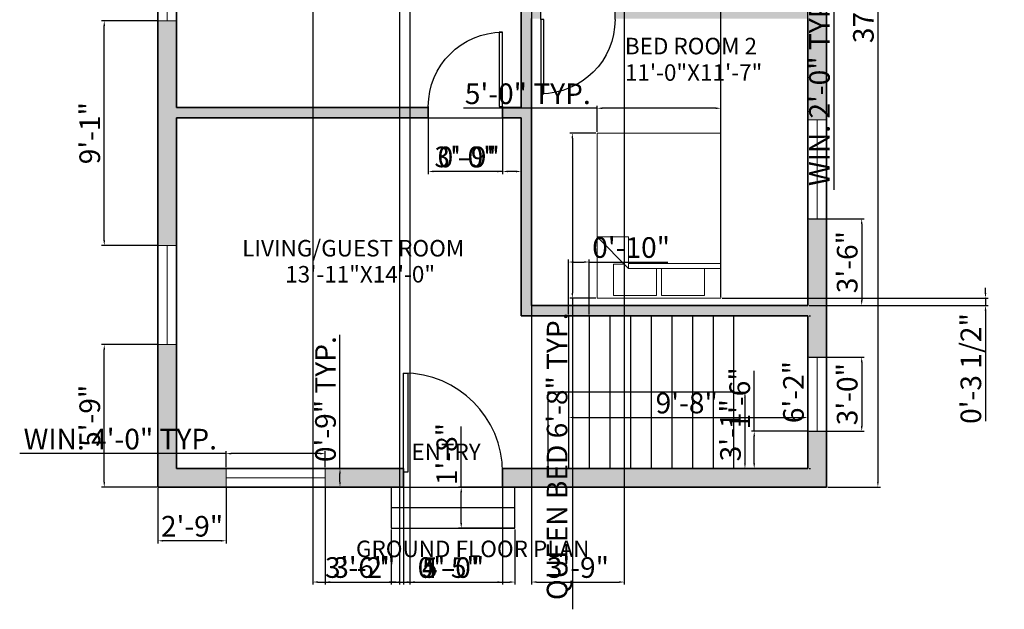
# Model space of a CAD drawing. Units: inches. Extents: x 3647 to 4124, y 1633 to 2205.
# Tile 1 of 3: x 3647 to 4124, y 1633 to 1919. Entities that reach past the tile are written whole.
import ezdxf

# ---------------------------------------------------------------- set-up
doc = ezdxf.new("R2010")
doc.units = ezdxf.units.IN
for name, color, linetype, lineweight in [('A-ANNO-DIMS', 2, 'Continuous', 18), ('A-ANNO-TEXT', 3, 'Continuous', 25), ('A-AREA-IDEN', 3, 'Continuous', 18), ('A-FURN', 8, 'Continuous', 18), ('DOOR', 6, 'Continuous', 25), ('STAIRS', 1, 'Continuous', 25), ('WALL', 42, 'Continuous', 35), ('WINDOW', 4, 'Continuous', 18)]:
    doc.layers.add(name, color=color, linetype=linetype, lineweight=lineweight)
doc.layers.add('A-WALL-PATT', color=18, linetype='Continuous', lineweight=13, true_color=0x000000)
doc.styles.get("Standard").update_dxf_attribs({"font": 'arial.ttf'})
doc.dimstyles.new('ISO-25', dxfattribs={"dimtxt": 10, "dimasz": 2.5, "dimexe": 1.25, "dimexo": 0.625, "dimtad": 1, "dimdec": 1, "dimlunit": 3, "dimtxsty": 'Standard', "dimcen": 2.5, "dimadec": 0, "dimazin": 0, "dimtfac": 1, "dimtdec": 1, "dimtmove": 0, "dimatfit": 3, "dimfxl": 1, "dimarcsym": 0})

# ---------------------------------------------------------------- blocks, each defined once
blk = doc.blocks.new('*U2')
for p, q in [((0, 0), (0, -6)), ((40, 0), (40, -6))]:
    blk.add_line(p, q)
blk.add_lwpolyline([(0, 0), (0, 40), (1.75, 40), (1.75, 0)], close=True)
blk.add_arc((0, 0), 40, 0, 90)
blk = doc.blocks.new('Bed - Queen')
for p, q in [((0, -80.00003), (0, 0)), ((0, 0), (59.99999, 0)), ((59.99999, 0), (59.99999, -80.00003)), ((7.99999, -1.2), (28.79998, -1.2)), ((7.99999, -14.4), (7.99999, -1.2)), ((28.79998, -1.2), (28.79998, -14.4)), ((31.19999, -1.2), (51.99999, -1.2)), ((31.19999, -14.4), (31.19999, -1.2)), ((51.99999, -1.2), (51.99999, -16.4)), ((0, -14.4), (44.8, -14.4)), ((44.8, -16.8), (0, -16.8)), ((59.99999, -29.6), (44.8, -14.4)), ((44.8, -14.4), (44.8, -29.6)), ((51.99999, -16.4), (46.79936, -16.4)), ((44.8, -29.6), (59.99999, -29.6)), ((59.99999, -80.00003), (0, -80.00003))]:
    blk.add_line(p, q)
blk = doc.blocks.new('*D8')
at = {"layer": 'A-ANNO-DIMS', "color": 0, "lineweight": -2, "transparency": 16777216}
for p, q in [((4029.34, 1775.28), (4029.96, 1775.28)), ((4028.71, 1772.78), (4028.71, 1703.78)), ((4029.34, 1701.28), (4029.96, 1701.28))]:
    blk.add_line(p, q, dxfattribs=at)
at = {"layer": 'A-ANNO-DIMS', "color": 0, "transparency": 16777216}
for points in [[(4028.3, 1772.78), (4029.13, 1772.78), (4028.71, 1775.28)], [(4028.3, 1703.78), (4029.13, 1703.78), (4028.71, 1701.28)]]:
    blk.add_solid(points, dxfattribs=at)
at = {"layer": 'Defpoints', "color": 0, "transparency": 16777216}
for p in [(4028.71, 1775.28), (4028.71, 1701.28), (4028.71, 1701.28)]:
    blk.add_point(p, dxfattribs=at)
at = {"layer": 'A-ANNO-DIMS', "color": 0, "transparency": 16777216, "insert": (4022.98, 1738.28), "char_height": 10, "attachment_point": 5, "rotation": 90}
blk.add_mtext('6\'-2"', dxfattribs=at)
blk = doc.blocks.new('*D9')
at = {"layer": 'A-ANNO-DIMS', "color": 0, "lineweight": -2, "transparency": 16777216}
for p, q in [((3912.71, 1737.66), (3912.71, 1724.71)), ((4028.71, 1737.66), (4028.71, 1724.71)), ((3915.21, 1725.96), (4026.21, 1725.96))]:
    blk.add_line(p, q, dxfattribs=at)
at = {"layer": 'A-ANNO-DIMS', "color": 0, "transparency": 16777216}
for points in [[(3915.21, 1726.38), (3915.21, 1725.54), (3912.71, 1725.96)], [(4026.21, 1726.38), (4026.21, 1725.54), (4028.71, 1725.96)]]:
    blk.add_solid(points, dxfattribs=at)
at = {"layer": 'Defpoints', "color": 0, "transparency": 16777216}
for p in [(3912.71, 1738.28), (4028.71, 1738.28), (4028.71, 1725.96)]:
    blk.add_point(p, dxfattribs=at)
at = {"layer": 'A-ANNO-DIMS', "color": 0, "transparency": 16777216, "insert": (3969.95, 1731.69), "char_height": 10, "attachment_point": 5}
blk.add_mtext('9\'-8"', dxfattribs=at)
blk = doc.blocks.new('*D10')
at = {"layer": 'A-ANNO-DIMS', "color": 0, "lineweight": -2, "transparency": 16777216}
for p, q in [((3993.34, 1738.28), (3999.44, 1738.28)), ((3998.19, 1735.78), (3998.19, 1703.78)), ((3993.34, 1701.28), (3999.44, 1701.28))]:
    blk.add_line(p, q, dxfattribs=at)
at = {"layer": 'A-ANNO-DIMS', "color": 0, "transparency": 16777216}
for points in [[(3997.78, 1735.78), (3998.61, 1735.78), (3998.19, 1738.28)], [(3997.78, 1703.78), (3998.61, 1703.78), (3998.19, 1701.28)]]:
    blk.add_solid(points, dxfattribs=at)
at = {"layer": 'Defpoints', "color": 0, "transparency": 16777216}
for p in [(3992.71, 1738.28), (3992.71, 1701.28), (3998.19, 1701.28)]:
    blk.add_point(p, dxfattribs=at)
at = {"layer": 'A-ANNO-DIMS', "color": 0, "transparency": 16777216, "insert": (3992.46, 1719.78), "char_height": 10, "attachment_point": 5, "rotation": 90}
blk.add_mtext('3\'-1"', dxfattribs=at)
blk = doc.blocks.new('*D12')
at = {"layer": 'A-ANNO-DIMS', "color": 0, "lineweight": -2, "transparency": 16777216}
for p, q in [((4038.34, 2136.28), (4063.86, 2136.28)), ((4062.61, 2133.78), (4062.61, 1694.78)), ((4038.34, 1692.28), (4063.86, 1692.28))]:
    blk.add_line(p, q, dxfattribs=at)
at = {"layer": 'A-ANNO-DIMS', "color": 0, "transparency": 16777216}
for points in [[(4062.19, 2133.78), (4063.02, 2133.78), (4062.61, 2136.28)], [(4062.19, 1694.78), (4063.02, 1694.78), (4062.61, 1692.28)]]:
    blk.add_solid(points, dxfattribs=at)
at = {"layer": 'Defpoints', "color": 0, "transparency": 16777216}
for p in [(4037.71, 2136.28), (4037.71, 1692.28), (4062.61, 1692.28)]:
    blk.add_point(p, dxfattribs=at)
at = {"layer": 'A-ANNO-DIMS', "color": 0, "transparency": 16777216, "insert": (4056.87, 1916.88), "char_height": 10, "attachment_point": 5, "rotation": 90}
blk.add_mtext("37'", dxfattribs=at)
blk = doc.blocks.new('WIN-48IN')
for p, q in [((9, 48), (0, 48)), ((4.5, 48), (4.5, 0)), ((9, 0), (0, 0))]:
    blk.add_line(p, q)
blk = doc.blocks.new('*D15')
at = {"layer": 'A-ANNO-DIMS', "color": 0, "lineweight": -2, "transparency": 16777216}
for p, q in [((3746.71, 1708.48), (3646.68, 1708.48)), ((3746.71, 1701.91), (3746.71, 1709.73)), ((3792.21, 1708.48), (3749.21, 1708.48)), ((3794.71, 1701.91), (3794.71, 1709.73))]:
    blk.add_line(p, q, dxfattribs=at)
at = {"layer": 'A-ANNO-DIMS', "color": 0, "transparency": 16777216}
for points in [[(3749.21, 1708.9), (3749.21, 1708.06), (3746.71, 1708.48)], [(3792.21, 1708.9), (3792.21, 1708.06), (3794.71, 1708.48)]]:
    blk.add_solid(points, dxfattribs=at)
at = {"layer": 'Defpoints', "color": 0, "transparency": 16777216}
for p in [(3746.71, 1708.48), (3746.71, 1701.28), (3794.71, 1701.28)]:
    blk.add_point(p, dxfattribs=at)
at = {"layer": 'A-ANNO-DIMS', "color": 0, "transparency": 16777216, "insert": (3695.45, 1714.21), "char_height": 10, "attachment_point": 5}
blk.add_mtext('WIN. 4\'-0" TYP.', dxfattribs=at)
blk = doc.blocks.new('*D16')
at = {"layer": 'A-ANNO-DIMS', "color": 0, "lineweight": -2, "transparency": 16777216}
for p, q in [((3801.91, 1701.28), (3801.91, 1765.99)), ((3795.34, 1701.28), (3803.16, 1701.28)), ((3801.91, 1694.78), (3801.91, 1698.78)), ((3795.34, 1692.28), (3803.16, 1692.28))]:
    blk.add_line(p, q, dxfattribs=at)
at = {"layer": 'A-ANNO-DIMS', "color": 0, "transparency": 16777216}
for points in [[(3801.5, 1698.78), (3802.33, 1698.78), (3801.91, 1701.28)], [(3801.5, 1694.78), (3802.33, 1694.78), (3801.91, 1692.28)]]:
    blk.add_solid(points, dxfattribs=at)
at = {"layer": 'Defpoints', "color": 0, "transparency": 16777216}
for p in [(3794.71, 1701.28), (3801.91, 1701.28), (3794.71, 1692.28)]:
    blk.add_point(p, dxfattribs=at)
at = {"layer": 'A-ANNO-DIMS', "color": 0, "transparency": 16777216, "insert": (3796.18, 1734.88), "char_height": 10, "attachment_point": 5, "rotation": 90}
blk.add_mtext('0\'-9" TYP.', dxfattribs=at)
blk = doc.blocks.new('*D17')
at = {"layer": 'A-ANNO-DIMS', "color": 0, "lineweight": -2, "transparency": 16777216}
for p, q in [((4038.34, 1960.28), (4042.56, 1960.28)), ((4041.31, 1957.78), (4041.31, 1938.78)), ((4038.34, 1936.28), (4042.56, 1936.28)), ((4041.31, 1936.28), (4041.31, 1836.25))]:
    blk.add_line(p, q, dxfattribs=at)
at = {"layer": 'A-ANNO-DIMS', "color": 0, "transparency": 16777216}
for points in [[(4040.9, 1957.78), (4041.73, 1957.78), (4041.31, 1960.28)], [(4040.9, 1938.78), (4041.73, 1938.78), (4041.31, 1936.28)]]:
    blk.add_solid(points, dxfattribs=at)
at = {"layer": 'Defpoints', "color": 0, "transparency": 16777216}
for p in [(4037.71, 1960.28), (4037.71, 1936.28), (4041.31, 1936.28)]:
    blk.add_point(p, dxfattribs=at)
at = {"layer": 'A-ANNO-DIMS', "color": 0, "transparency": 16777216, "insert": (4035.58, 1885.02), "char_height": 10, "attachment_point": 5, "rotation": 90}
blk.add_mtext('WIN. 2\'-0" TYP.', dxfattribs=at)
blk = doc.blocks.new('*D19')
at = {"layer": 'A-ANNO-DIMS', "color": 0, "lineweight": -2, "transparency": 16777216}
for p, q in [((3925.91, 1863.86), (3913.28, 1863.86)), ((3914.53, 1861.36), (3914.53, 1786.36)), ((3925.91, 1783.86), (3913.28, 1783.86)), ((3914.53, 1783.86), (3914.53, 1633.01))]:
    blk.add_line(p, q, dxfattribs=at)
at = {"layer": 'A-ANNO-DIMS', "color": 0, "transparency": 16777216}
for points in [[(3914.12, 1861.36), (3914.95, 1861.36), (3914.53, 1863.86)], [(3914.12, 1786.36), (3914.95, 1786.36), (3914.53, 1783.86)]]:
    blk.add_solid(points, dxfattribs=at)
at = {"layer": 'Defpoints', "color": 0, "transparency": 16777216}
for p in [(3926.53, 1863.86), (3914.53, 1783.86), (3926.53, 1783.86)]:
    blk.add_point(p, dxfattribs=at)
at = {"layer": 'A-ANNO-DIMS', "color": 0, "transparency": 16777216, "insert": (3908.43, 1707.19), "char_height": 10, "attachment_point": 5, "rotation": 90}
blk.add_mtext('QUEEN BED 6\'-8" TYP.', dxfattribs=at)
blk = doc.blocks.new('*D20')
at = {"layer": 'A-ANNO-DIMS', "color": 0, "lineweight": -2, "transparency": 16777216}
for p, q in [((3926.53, 1875.86), (3861.83, 1875.86)), ((3926.53, 1864.49), (3926.53, 1877.11)), ((3984.03, 1875.86), (3929.03, 1875.86)), ((3986.53, 1864.49), (3986.53, 1877.11))]:
    blk.add_line(p, q, dxfattribs=at)
at = {"layer": 'A-ANNO-DIMS', "color": 0, "transparency": 16777216}
for points in [[(3929.03, 1876.28), (3929.03, 1875.45), (3926.53, 1875.86)], [(3984.03, 1876.28), (3984.03, 1875.45), (3986.53, 1875.86)]]:
    blk.add_solid(points, dxfattribs=at)
at = {"layer": 'Defpoints', "color": 0, "transparency": 16777216}
for p in [(3926.53, 1875.86), (3926.53, 1863.86), (3986.53, 1863.86)]:
    blk.add_point(p, dxfattribs=at)
at = {"layer": 'A-ANNO-DIMS', "color": 0, "transparency": 16777216, "insert": (3892.93, 1881.59), "char_height": 10, "attachment_point": 5}
blk.add_mtext('5\'-0" TYP.', dxfattribs=at)
blk = doc.blocks.new('*D28')
at = {"layer": 'A-ANNO-DIMS', "color": 0, "lineweight": -2, "transparency": 16777216}
for p, q in [((3844.71, 1870.66), (3844.71, 1843.98)), ((3880.71, 1870.66), (3880.71, 1843.98)), ((3878.21, 1845.23), (3847.21, 1845.23))]:
    blk.add_line(p, q, dxfattribs=at)
at = {"layer": 'A-ANNO-DIMS', "color": 0, "transparency": 16777216}
for points in [[(3847.21, 1845.65), (3847.21, 1844.81), (3844.71, 1845.23)], [(3878.21, 1845.65), (3878.21, 1844.81), (3880.71, 1845.23)]]:
    blk.add_solid(points, dxfattribs=at)
at = {"layer": 'Defpoints', "color": 0, "transparency": 16777216}
for p in [(3844.71, 1871.28), (3880.71, 1871.28), (3844.71, 1845.23)]:
    blk.add_point(p, dxfattribs=at)
at = {"layer": 'A-ANNO-DIMS', "color": 0, "transparency": 16777216, "insert": (3862.71, 1850.97), "char_height": 10, "attachment_point": 5}
blk.add_mtext('3\'-0"', dxfattribs=at)
blk = doc.blocks.new('*D30')
at = {"layer": 'A-ANNO-DIMS', "color": 0, "lineweight": -2, "transparency": 16777216}
for p, q in [((3894.71, 1989.66), (3894.71, 1644.98)), ((3939.71, 1989.66), (3939.71, 1644.98)), ((3897.21, 1646.23), (3937.21, 1646.23))]:
    blk.add_line(p, q, dxfattribs=at)
at = {"layer": 'A-ANNO-DIMS', "color": 0, "transparency": 16777216}
for points in [[(3897.21, 1646.65), (3897.21, 1645.81), (3894.71, 1646.23)], [(3937.21, 1646.65), (3937.21, 1645.81), (3939.71, 1646.23)]]:
    blk.add_solid(points, dxfattribs=at)
at = {"layer": 'Defpoints', "color": 0, "transparency": 16777216}
for p in [(3894.71, 1990.28), (3939.71, 1990.28), (3939.71, 1646.23)]:
    blk.add_point(p, dxfattribs=at)
at = {"layer": 'A-ANNO-DIMS', "color": 0, "transparency": 16777216, "insert": (3917.21, 1651.97), "char_height": 10, "attachment_point": 5}
blk.add_mtext('3\'-9"', dxfattribs=at)
blk = doc.blocks.new('*D31')
at = {"layer": 'A-ANNO-DIMS', "color": 0, "lineweight": -2, "transparency": 16777216}
for p, q in [((3788.71, 2013.66), (3788.71, 1644.98)), ((3830.71, 2013.66), (3830.71, 1644.98)), ((3791.21, 1646.23), (3828.21, 1646.23))]:
    blk.add_line(p, q, dxfattribs=at)
at = {"layer": 'A-ANNO-DIMS', "color": 0, "transparency": 16777216}
for points in [[(3791.21, 1646.65), (3791.21, 1645.81), (3788.71, 1646.23)], [(3828.21, 1646.65), (3828.21, 1645.81), (3830.71, 1646.23)]]:
    blk.add_solid(points, dxfattribs=at)
at = {"layer": 'Defpoints', "color": 0, "transparency": 16777216}
for p in [(3788.71, 2014.28), (3830.71, 2014.28), (3830.71, 1646.23)]:
    blk.add_point(p, dxfattribs=at)
at = {"layer": 'A-ANNO-DIMS', "color": 0, "transparency": 16777216, "insert": (3809.71, 1651.97), "char_height": 10, "attachment_point": 5}
blk.add_mtext('3\'-6"', dxfattribs=at)
blk = doc.blocks.new('*D32')
at = {"layer": 'A-ANNO-DIMS', "color": 0, "lineweight": -2, "transparency": 16777216}
for p, q in [((3830.71, 2126.66), (3830.71, 1644.98)), ((3835.71, 2126.66), (3835.71, 1644.98)), ((3828.21, 1646.23), (3825.71, 1646.23)), ((3830.71, 1646.23), (3835.71, 1646.23)), ((3838.21, 1646.23), (3868.55, 1646.23))]:
    blk.add_line(p, q, dxfattribs=at)
at = {"layer": 'A-ANNO-DIMS', "color": 0, "transparency": 16777216}
for points in [[(3828.21, 1646.65), (3828.21, 1645.81), (3830.71, 1646.23)], [(3838.21, 1646.65), (3838.21, 1645.81), (3835.71, 1646.23)]]:
    blk.add_solid(points, dxfattribs=at)
at = {"layer": 'Defpoints', "color": 0, "transparency": 16777216}
for p in [(3830.71, 2127.28), (3835.71, 2127.28), (3835.71, 1646.23)]:
    blk.add_point(p, dxfattribs=at)
at = {"layer": 'A-ANNO-DIMS', "color": 0, "transparency": 16777216, "insert": (3854.63, 1651.96), "char_height": 10, "attachment_point": 5}
blk.add_mtext('0\'-5"', dxfattribs=at)
blk = doc.blocks.new('*D33')
at = {"layer": 'A-ANNO-DIMS', "color": 0, "lineweight": -2, "transparency": 16777216}
for p, q in [((3713.71, 1691.66), (3713.71, 1664.98)), ((3746.71, 1691.66), (3746.71, 1664.98)), ((3744.21, 1666.23), (3716.21, 1666.23))]:
    blk.add_line(p, q, dxfattribs=at)
at = {"layer": 'A-ANNO-DIMS', "color": 0, "transparency": 16777216}
for points in [[(3716.21, 1666.65), (3716.21, 1665.81), (3713.71, 1666.23)], [(3744.21, 1666.65), (3744.21, 1665.81), (3746.71, 1666.23)]]:
    blk.add_solid(points, dxfattribs=at)
at = {"layer": 'Defpoints', "color": 0, "transparency": 16777216}
for p in [(3713.71, 1692.28), (3746.71, 1692.28), (3713.71, 1666.23)]:
    blk.add_point(p, dxfattribs=at)
at = {"layer": 'A-ANNO-DIMS', "color": 0, "transparency": 16777216, "insert": (3730.21, 1671.96), "char_height": 10, "attachment_point": 5}
blk.add_mtext('2\'-9"', dxfattribs=at)
blk = doc.blocks.new('*D34')
at = {"layer": 'A-ANNO-DIMS', "color": 0, "lineweight": -2, "transparency": 16777216}
for p, q in [((3794.71, 1691.66), (3794.71, 1644.98)), ((3832.71, 1691.66), (3832.71, 1644.98)), ((3797.21, 1646.23), (3830.21, 1646.23))]:
    blk.add_line(p, q, dxfattribs=at)
at = {"layer": 'A-ANNO-DIMS', "color": 0, "transparency": 16777216}
for points in [[(3797.21, 1646.65), (3797.21, 1645.81), (3794.71, 1646.23)], [(3830.21, 1646.65), (3830.21, 1645.81), (3832.71, 1646.23)]]:
    blk.add_solid(points, dxfattribs=at)
at = {"layer": 'Defpoints', "color": 0, "transparency": 16777216}
for p in [(3794.71, 1692.28), (3832.71, 1692.28), (3832.71, 1646.23)]:
    blk.add_point(p, dxfattribs=at)
at = {"layer": 'A-ANNO-DIMS', "color": 0, "transparency": 16777216, "insert": (3813.71, 1651.97), "char_height": 10, "attachment_point": 5}
blk.add_mtext('3\'-2"', dxfattribs=at)
blk = doc.blocks.new('*D35')
at = {"layer": 'A-ANNO-DIMS', "color": 0, "lineweight": -2, "transparency": 16777216}
for p, q in [((3832.71, 1691.66), (3832.71, 1644.98)), ((3880.71, 1691.66), (3880.71, 1644.98)), ((3835.21, 1646.23), (3878.21, 1646.23))]:
    blk.add_line(p, q, dxfattribs=at)
at = {"layer": 'A-ANNO-DIMS', "color": 0, "transparency": 16777216}
for points in [[(3835.21, 1646.65), (3835.21, 1645.81), (3832.71, 1646.23)], [(3878.21, 1646.65), (3878.21, 1645.81), (3880.71, 1646.23)]]:
    blk.add_solid(points, dxfattribs=at)
at = {"layer": 'Defpoints', "color": 0, "transparency": 16777216}
for p in [(3832.71, 1692.28), (3880.71, 1692.28), (3880.71, 1646.23)]:
    blk.add_point(p, dxfattribs=at)
at = {"layer": 'A-ANNO-DIMS', "color": 0, "transparency": 16777216, "insert": (3856.71, 1651.96), "char_height": 10, "attachment_point": 5}
blk.add_mtext('4\'-0"', dxfattribs=at)
blk = doc.blocks.new('*D36')
at = {"layer": 'A-ANNO-DIMS', "color": 0, "lineweight": -2, "transparency": 16777216}
for p, q in [((3826.71, 1671.66), (3826.71, 1644.98)), ((3886.71, 1671.66), (3886.71, 1644.98)), ((3829.21, 1646.23), (3884.21, 1646.23))]:
    blk.add_line(p, q, dxfattribs=at)
at = {"layer": 'A-ANNO-DIMS', "color": 0, "transparency": 16777216}
for points in [[(3829.21, 1646.65), (3829.21, 1645.81), (3826.71, 1646.23)], [(3884.21, 1646.65), (3884.21, 1645.81), (3886.71, 1646.23)]]:
    blk.add_solid(points, dxfattribs=at)
at = {"layer": 'Defpoints', "color": 0, "transparency": 16777216}
for p in [(3826.71, 1672.28), (3886.71, 1672.28), (3886.71, 1646.23)]:
    blk.add_point(p, dxfattribs=at)
at = {"layer": 'A-ANNO-DIMS', "color": 0, "transparency": 16777216, "insert": (3856.71, 1651.96), "char_height": 10, "attachment_point": 5}
blk.add_mtext('5\'-0"', dxfattribs=at)
blk = doc.blocks.new('*D37')
at = {"layer": 'A-ANNO-DIMS', "color": 0, "lineweight": -2, "transparency": 16777216}
for p, q in [((3860.66, 1692.28), (3860.66, 1721.67)), ((3886.09, 1692.28), (3859.41, 1692.28)), ((3860.66, 1674.78), (3860.66, 1689.78)), ((3886.09, 1672.28), (3859.41, 1672.28))]:
    blk.add_line(p, q, dxfattribs=at)
at = {"layer": 'A-ANNO-DIMS', "color": 0, "transparency": 16777216}
for points in [[(3860.25, 1689.78), (3861.08, 1689.78), (3860.66, 1692.28)], [(3860.25, 1674.78), (3861.08, 1674.78), (3860.66, 1672.28)]]:
    blk.add_solid(points, dxfattribs=at)
at = {"layer": 'Defpoints', "color": 0, "transparency": 16777216}
for p in [(3860.66, 1692.28), (3886.71, 1692.28), (3886.71, 1672.28)]:
    blk.add_point(p, dxfattribs=at)
at = {"layer": 'A-ANNO-DIMS', "color": 0, "transparency": 16777216, "insert": (3854.93, 1708.23), "char_height": 10, "attachment_point": 5, "rotation": 90}
blk.add_mtext('1\'-8"', dxfattribs=at)
blk = doc.blocks.new('*D38')
at = {"layer": 'A-ANNO-DIMS', "color": 0, "lineweight": -2, "transparency": 16777216}
for p, q in [((3713.09, 1761.28), (3686.41, 1761.28)), ((3687.66, 1694.78), (3687.66, 1758.78)), ((3713.09, 1692.28), (3686.41, 1692.28))]:
    blk.add_line(p, q, dxfattribs=at)
at = {"layer": 'A-ANNO-DIMS', "color": 0, "transparency": 16777216}
for points in [[(3687.25, 1758.78), (3688.08, 1758.78), (3687.66, 1761.28)], [(3687.25, 1694.78), (3688.08, 1694.78), (3687.66, 1692.28)]]:
    blk.add_solid(points, dxfattribs=at)
at = {"layer": 'Defpoints', "color": 0, "transparency": 16777216}
for p in [(3687.66, 1761.28), (3713.71, 1761.28), (3713.71, 1692.28)]:
    blk.add_point(p, dxfattribs=at)
at = {"layer": 'A-ANNO-DIMS', "color": 0, "transparency": 16777216, "insert": (3681.93, 1726.78), "char_height": 10, "attachment_point": 5, "rotation": 90}
blk.add_mtext('5\'-9"', dxfattribs=at)
blk = doc.blocks.new('*D39')
at = {"layer": 'A-ANNO-DIMS', "color": 0, "lineweight": -2, "transparency": 16777216}
for p, q in [((3713.09, 1918.28), (3686.41, 1918.28)), ((3687.66, 1811.78), (3687.66, 1915.78)), ((3713.09, 1809.28), (3686.41, 1809.28))]:
    blk.add_line(p, q, dxfattribs=at)
at = {"layer": 'A-ANNO-DIMS', "color": 0, "transparency": 16777216}
for points in [[(3687.25, 1915.78), (3688.08, 1915.78), (3687.66, 1918.28)], [(3687.25, 1811.78), (3688.08, 1811.78), (3687.66, 1809.28)]]:
    blk.add_solid(points, dxfattribs=at)
at = {"layer": 'Defpoints', "color": 0, "transparency": 16777216}
for p in [(3687.66, 1918.28), (3713.71, 1918.28), (3713.71, 1809.28)]:
    blk.add_point(p, dxfattribs=at)
at = {"layer": 'A-ANNO-DIMS', "color": 0, "transparency": 16777216, "insert": (3681.93, 1863.78), "char_height": 10, "attachment_point": 5, "rotation": 90}
blk.add_mtext('9\'-1"', dxfattribs=at)
blk = doc.blocks.new('*D44')
at = {"layer": 'A-ANNO-DIMS', "color": 0, "lineweight": -2, "transparency": 16777216}
for p, q in [((4029.34, 1822.28), (4056.01, 1822.28)), ((4054.76, 1819.78), (4054.76, 1782.78)), ((4029.34, 1780.28), (4056.01, 1780.28))]:
    blk.add_line(p, q, dxfattribs=at)
at = {"layer": 'A-ANNO-DIMS', "color": 0, "transparency": 16777216}
for points in [[(4054.35, 1819.78), (4055.18, 1819.78), (4054.76, 1822.28)], [(4054.35, 1782.78), (4055.18, 1782.78), (4054.76, 1780.28)]]:
    blk.add_solid(points, dxfattribs=at)
at = {"layer": 'Defpoints', "color": 0, "transparency": 16777216}
for p in [(4028.71, 1822.28), (4028.71, 1780.28), (4054.76, 1780.28)]:
    blk.add_point(p, dxfattribs=at)
at = {"layer": 'A-ANNO-DIMS', "color": 0, "transparency": 16777216, "insert": (4049.03, 1801.28), "char_height": 10, "attachment_point": 5, "rotation": 90}
blk.add_mtext('3\'-6"', dxfattribs=at)
blk = doc.blocks.new('*D45')
at = {"layer": 'A-ANNO-DIMS', "color": 0, "lineweight": -2, "transparency": 16777216}
for p, q in [((4002.66, 1719.28), (4002.66, 1748.67)), ((4028.09, 1719.28), (4001.41, 1719.28)), ((4002.66, 1703.78), (4002.66, 1716.78)), ((4028.09, 1701.28), (4001.41, 1701.28))]:
    blk.add_line(p, q, dxfattribs=at)
at = {"layer": 'A-ANNO-DIMS', "color": 0, "transparency": 16777216}
for points in [[(4002.25, 1716.78), (4003.08, 1716.78), (4002.66, 1719.28)], [(4002.25, 1703.78), (4003.08, 1703.78), (4002.66, 1701.28)]]:
    blk.add_solid(points, dxfattribs=at)
at = {"layer": 'Defpoints', "color": 0, "transparency": 16777216}
for p in [(4002.66, 1719.28), (4028.71, 1719.28), (4028.71, 1701.28)]:
    blk.add_point(p, dxfattribs=at)
at = {"layer": 'A-ANNO-DIMS', "color": 0, "transparency": 16777216, "insert": (3996.93, 1735.23), "char_height": 10, "attachment_point": 5, "rotation": 90}
blk.add_mtext('1\'-6"', dxfattribs=at)
blk = doc.blocks.new('*D46')
at = {"layer": 'A-ANNO-DIMS', "color": 0, "lineweight": -2, "transparency": 16777216}
for p, q in [((4029.34, 1755.28), (4056.01, 1755.28)), ((4054.76, 1752.78), (4054.76, 1721.78)), ((4029.34, 1719.28), (4056.01, 1719.28))]:
    blk.add_line(p, q, dxfattribs=at)
at = {"layer": 'A-ANNO-DIMS', "color": 0, "transparency": 16777216}
for points in [[(4054.35, 1752.78), (4055.18, 1752.78), (4054.76, 1755.28)], [(4054.35, 1721.78), (4055.18, 1721.78), (4054.76, 1719.28)]]:
    blk.add_solid(points, dxfattribs=at)
at = {"layer": 'Defpoints', "color": 0, "transparency": 16777216}
for p in [(4028.71, 1755.28), (4028.71, 1719.28), (4054.76, 1719.28)]:
    blk.add_point(p, dxfattribs=at)
at = {"layer": 'A-ANNO-DIMS', "color": 0, "transparency": 16777216, "insert": (4049.03, 1737.28), "char_height": 10, "attachment_point": 5, "rotation": 90}
blk.add_mtext('3\'-0"', dxfattribs=at)
blk = doc.blocks.new('*D47')
at = {"layer": 'A-ANNO-DIMS', "color": 0, "lineweight": -2, "transparency": 16777216}
for p, q in [((3880.71, 1870.66), (3880.71, 1843.98)), ((3889.71, 1870.66), (3889.71, 1843.98)), ((3880.71, 1845.23), (3850.38, 1845.23)), ((3887.21, 1845.23), (3883.21, 1845.23))]:
    blk.add_line(p, q, dxfattribs=at)
at = {"layer": 'A-ANNO-DIMS', "color": 0, "transparency": 16777216}
for points in [[(3883.21, 1845.65), (3883.21, 1844.81), (3880.71, 1845.23)], [(3887.21, 1845.65), (3887.21, 1844.81), (3889.71, 1845.23)]]:
    blk.add_solid(points, dxfattribs=at)
at = {"layer": 'Defpoints', "color": 0, "transparency": 16777216}
for p in [(3880.71, 1871.28), (3889.71, 1871.28), (3880.71, 1845.23)]:
    blk.add_point(p, dxfattribs=at)
at = {"layer": 'A-ANNO-DIMS', "color": 0, "transparency": 16777216, "insert": (3864.3, 1850.96), "char_height": 10, "attachment_point": 5}
blk.add_mtext('0\'-9"', dxfattribs=at)
blk = doc.blocks.new('*D51')
at = {"layer": 'A-ANNO-DIMS', "color": 0, "lineweight": -2, "transparency": 16777216}
for p, q in [((3912.71, 1775.91), (3912.71, 1802.58)), ((3915.21, 1801.33), (3920.21, 1801.33)), ((3922.71, 1775.91), (3922.71, 1802.58)), ((3922.71, 1801.33), (3960.82, 1801.33))]:
    blk.add_line(p, q, dxfattribs=at)
at = {"layer": 'A-ANNO-DIMS', "color": 0, "transparency": 16777216}
for points in [[(3915.21, 1801.75), (3915.21, 1800.91), (3912.71, 1801.33)], [(3920.21, 1801.75), (3920.21, 1800.91), (3922.71, 1801.33)]]:
    blk.add_solid(points, dxfattribs=at)
at = {"layer": 'Defpoints', "color": 0, "transparency": 16777216}
for p in [(3922.71, 1801.33), (3912.71, 1775.28), (3922.71, 1775.28)]:
    blk.add_point(p, dxfattribs=at)
at = {"layer": 'A-ANNO-DIMS', "color": 0, "transparency": 16777216, "insert": (3943.01, 1807.06), "char_height": 10, "attachment_point": 5}
blk.add_mtext('0\'-10"', dxfattribs=at)
blk = doc.blocks.new('*D60')
at = {"layer": 'A-ANNO-DIMS', "color": 0, "lineweight": -2, "transparency": 16777216}
for p, q in [((3986.53, 1784.49), (3986.53, 2163.58)), ((3989.03, 2162.33), (4026.21, 2162.33)), ((4028.71, 1780.91), (4028.71, 2163.58))]:
    blk.add_line(p, q, dxfattribs=at)
at = {"layer": 'A-ANNO-DIMS', "color": 0, "transparency": 16777216}
for points in [[(3989.03, 2162.75), (3989.03, 2161.91), (3986.53, 2162.33)], [(4026.21, 2162.75), (4026.21, 2161.91), (4028.71, 2162.33)]]:
    blk.add_solid(points, dxfattribs=at)
at = {"layer": 'Defpoints', "color": 0, "transparency": 16777216}
for p in [(4028.71, 2162.33), (3986.53, 1783.86), (4028.71, 1780.28)]:
    blk.add_point(p, dxfattribs=at)
at = {"layer": 'A-ANNO-DIMS', "color": 0, "transparency": 16777216, "insert": (4007.62, 2168.07), "char_height": 10, "attachment_point": 5}
blk.add_mtext('3\'-6"', dxfattribs=at)
blk = doc.blocks.new('*D61')
at = {"layer": 'A-ANNO-DIMS', "color": 0, "lineweight": -2, "transparency": 16777216}
for p, q in [((4114.76, 1786.36), (4114.76, 1788.86)), ((3987.16, 1783.86), (4116.01, 1783.86)), ((4029.34, 1780.28), (4116.01, 1780.28)), ((4114.76, 1783.86), (4114.76, 1780.28)), ((4114.76, 1777.78), (4114.76, 1724.15))]:
    blk.add_line(p, q, dxfattribs=at)
at = {"layer": 'A-ANNO-DIMS', "color": 0, "transparency": 16777216}
for points in [[(4114.35, 1786.36), (4115.18, 1786.36), (4114.76, 1783.86)], [(4114.35, 1777.78), (4115.18, 1777.78), (4114.76, 1780.28)]]:
    blk.add_solid(points, dxfattribs=at)
at = {"layer": 'Defpoints', "color": 0, "transparency": 16777216}
for p in [(3986.53, 1783.86), (4028.71, 1780.28), (4114.76, 1780.28)]:
    blk.add_point(p, dxfattribs=at)
at = {"layer": 'A-ANNO-DIMS', "color": 0, "transparency": 16777216, "insert": (4108.96, 1749.71), "char_height": 10, "attachment_point": 5, "rotation": 90}
blk.add_mtext('0\'-3 1/2"', dxfattribs=at)

msp = doc.modelspace()

# ---------------------------------------------------------------- hatches: boundary and pattern name
at = {"layer": 'A-WALL-PATT'}
h = msp.add_hatch(color=256, dxfattribs=at)
h.dxf.hatch_style = 1
h.paths.add_polyline_path([(4037.71, 1936.28), (4028.71, 1936.28), (4028.71, 1924.28), (3944.71, 1924.28), (3944.71, 1957.28), (3939.71, 1957.28), (3939.71, 1924.28), (3935.21, 1924.28), (3935.21, 1919.28), (4028.71, 1919.28), (4028.71, 1870.28), (4037.71, 1870.28)])
h = msp.add_hatch(color=256, dxfattribs=at)
h.dxf.hatch_style = 1
h.paths.add_polyline_path([(4037.71, 1822.28), (4028.71, 1822.28), (4028.71, 1780.28), (3894.71, 1780.28), (3894.71, 1919.28), (3899.21, 1919.28), (3899.21, 1924.28), (3894.71, 1924.28), (3894.71, 1945.28), (3889.71, 1945.28), (3889.71, 1876.28), (3880.71, 1876.28), (3880.71, 1871.28), (3889.71, 1871.28), (3889.71, 1775.28), (4028.71, 1775.28), (4028.71, 1755.28), (4037.71, 1755.28)])
h = msp.add_hatch(color=256, dxfattribs=at)
h.dxf.hatch_style = 1
h.paths.add_polyline_path([(3722.71, 1871.28), (3844.71, 1871.28), (3844.71, 1876.28), (3722.71, 1876.28), (3722.71, 1918.28), (3713.71, 1918.28), (3713.71, 1809.28), (3722.71, 1809.28)])
h = msp.add_hatch(color=256, dxfattribs=at)
h.dxf.hatch_style = 1
h.paths.add_polyline_path([(3746.71, 1701.28), (3722.71, 1701.28), (3722.71, 1761.28), (3713.71, 1761.28), (3713.71, 1692.28), (3746.71, 1692.28)])
h = msp.add_hatch(color=256, dxfattribs=at)
h.dxf.hatch_style = 1
h.paths.add_polyline_path([(4037.71, 1719.28), (4028.71, 1719.28), (4028.71, 1701.28), (3880.71, 1701.28), (3880.71, 1692.28), (4037.71, 1692.28)])
h = msp.add_hatch(color=256, dxfattribs=at)
h.dxf.hatch_style = 1
h.paths.add_polyline_path([(3832.71, 1699.48), (3832.71, 1701.28), (3794.71, 1701.28), (3794.71, 1692.28), (3832.71, 1692.28)])

# ---------------------------------------------------------------- linework, layer by layer
at = {"layer": 'DOOR'}
for p, q in [((3844.71, 1871.28), (3880.71, 1871.28)), ((3832.71, 1692.28), (3880.71, 1692.28))]:
    msp.add_line(p, q, dxfattribs=at)
at = {"layer": 'STAIRS'}
for p, q in [((3912.71, 1775.28), (3912.71, 1738.28)), ((3922.71, 1775.28), (3922.71, 1701.28)), ((3932.71, 1775.28), (3932.71, 1701.28)), ((3942.71, 1775.28), (3942.71, 1701.28)), ((3952.71, 1775.28), (3952.71, 1701.28)), ((3962.71, 1775.28), (3962.71, 1701.28)), ((3972.71, 1775.28), (3972.71, 1701.28)), ((3982.71, 1775.28), (3982.71, 1701.28)), ((3992.71, 1775.28), (3992.71, 1701.28)), ((3992.71, 1738.28), (3902.71, 1738.28)), ((3902.71, 1738.28), (3902.71, 1701.28)), ((3912.71, 1738.28), (3912.71, 1701.28)), ((3826.71, 1692.28), (3826.71, 1682.28)), ((3886.71, 1682.28), (3886.71, 1692.28)), ((3826.71, 1682.28), (3880.71, 1682.28)), ((3826.71, 1682.28), (3826.71, 1672.28)), ((3880.71, 1682.28), (3886.71, 1682.28)), ((3886.71, 1672.28), (3886.71, 1682.28)), ((3826.71, 1672.28), (3886.71, 1672.28))]:
    msp.add_line(p, q, dxfattribs=at)
at = {"layer": 'WALL'}
for p, q in [((3713.71, 1692.28), (3713.71, 2136.28)), ((4037.71, 2136.28), (4037.71, 1692.28)), ((3722.71, 1876.28), (3722.71, 2014.28)), ((3889.71, 1876.28), (3889.71, 1945.28)), ((3894.71, 1780.28), (3894.71, 1919.28)), ((4028.71, 1919.28), (4028.71, 1780.28)), ((3722.71, 1876.28), (3844.71, 1876.28)), ((3844.71, 1871.28), (3844.71, 1876.28)), ((3880.71, 1871.28), (3880.71, 1876.28)), ((3880.71, 1876.28), (3889.71, 1876.28)), ((3722.71, 1701.28), (3722.71, 1871.28)), ((3722.71, 1871.28), (3844.71, 1871.28)), ((3880.71, 1871.28), (3889.71, 1871.28)), ((3889.71, 1775.28), (3889.71, 1871.28)), ((3894.71, 1780.28), (4028.71, 1780.28)), ((3889.71, 1775.28), (4028.71, 1775.28)), ((4028.71, 1775.28), (4028.71, 1701.28)), ((3832.71, 1701.28), (3722.71, 1701.28)), ((3832.71, 1692.28), (3832.71, 1701.28)), ((4028.71, 1701.28), (3880.71, 1701.28)), ((3880.71, 1692.28), (3880.71, 1701.28)), ((3832.71, 1692.28), (3713.71, 1692.28)), ((4037.71, 1692.28), (3880.71, 1692.28))]:
    msp.add_line(p, q, dxfattribs=at)
at = {"layer": 'WINDOW'}
for p, q in [((4028.71, 1755.28), (4037.71, 1755.28)), ((4033.21, 1755.28), (4033.21, 1719.28)), ((4028.71, 1719.28), (4037.71, 1719.28))]:
    msp.add_line(p, q, dxfattribs=at)

# ---------------------------------------------------------------- block references
at = {"layer": 'A-FURN', "rotation": 180}
msp.add_blockref('Bed - Queen', (3986.53, 1783.86), dxfattribs=at)
at = {"layer": 'DOOR', "xscale": -0.9, "yscale": 0.9, "zscale": 0.9, "rotation": 180}
msp.add_blockref('*U2', (3899.21, 1918.88), dxfattribs=at)
at = {"layer": 'DOOR'}
for p, xscale, yscale, zscale in [((3880.71, 1876.68), -0.8999999999999886, 0.8999999999999886, 0.8999999999999886), ((3832.71, 1699.48), 1.199999999999988, 1.199999999999988, 1.199999999999988)]:
    msp.add_blockref('*U2', p, dxfattribs=dict(at, xscale=xscale, yscale=yscale, zscale=zscale))
at = {"layer": 'WINDOW'}
msp.add_blockref('WIN-48IN', (3713.71, 1918.28), dxfattribs=at)
for p, rotation in [((4037.71, 1870.28), 180), ((3722.71, 1809.28), 180), ((3794.71, 1692.28), 90.00000000000182)]:
    msp.add_blockref('WIN-48IN', p, dxfattribs=dict(at, rotation=rotation))

# ---------------------------------------------------------------- texts
at = {"layer": 'A-ANNO-TEXT'}
msp.add_text('GROUND FLOOR PLAN', height=8, dxfattribs=at).set_placement((3809.66, 1658.3))
at = {"layer": 'A-AREA-IDEN'}
for s, p in [('BED ROOM 2', (3939.98, 1902)), ('11\'-0"X11\'-7"', (3939.98, 1889.15)), ('LIVING/GUEST ROOM', (3754.51, 1804.02)), ('13\'-11"X14\'-0"', (3775.34, 1791.4)), ('ENTRY', (3836.53, 1705.35))]:
    msp.add_text(s, height=8, dxfattribs=at).set_placement(p)

# ---------------------------------------------------------------- dimensions: what is measured, and where the dimension line sits
at = {"layer": 'A-ANNO-DIMS'}
for base, p1, p2, picture, middle in [((4028.71, 2162.33), (3986.53, 1783.86), (4028.71, 1780.28), '*D60', (4007.62, 2168.07)), ((3835.71, 1646.23), (3830.71, 2127.28), (3835.71, 2127.28), '*D32', (3854.63, 1651.96)), ((3830.71, 1646.23), (3788.71, 2014.28), (3830.71, 2014.28), '*D31', (3809.71, 1651.97)), ((3939.71, 1646.23), (3894.71, 1990.28), (3939.71, 1990.28), '*D30', (3917.21, 1651.97)), ((3922.71, 1801.33), (3912.71, 1775.28), (3922.71, 1775.28), '*D51', (3943.01, 1807.06)), ((3832.71, 1646.23), (3794.71, 1692.28), (3832.71, 1692.28), '*D34', (3813.71, 1651.97)), ((3880.71, 1646.23), (3832.71, 1692.28), (3880.71, 1692.28), '*D35', (3856.71, 1651.96)), ((3886.71, 1646.23), (3826.71, 1672.28), (3886.71, 1672.28), '*D36', (3856.71, 1651.96))]:
    dim = msp.add_linear_dim(base=base, p1=p1, p2=p2, dimstyle='ISO-25', override={"dimdec": 1, "dimlfac": 1, "dimrnd": 0, "dimzin": 1, "dimdsep": 46, "dimlunit": 4, "dimfrac": 2}, dxfattribs=at)
    dim.commit()
    dim.dimension.update_dxf_attribs({"geometry": picture, "text_midpoint": middle})
dim = msp.add_linear_dim(base=(4062.61, 1692.28), p1=(4037.71, 2136.28), p2=(4037.71, 1692.28), angle=90, dimstyle='ISO-25', override={"dimclrd": 0, "dimclre": 0, "dimclrt": 0}, dxfattribs=at)
dim.commit()
dim.dimension.update_dxf_attribs({"geometry": '*D12', "text_midpoint": (4062.61, 1916.88), "dimtype": 160})
for base, p1, p2, angle, text, picture, middle in [((4041.31, 1936.28), (4037.71, 1960.28), (4037.71, 1936.28), 270, 'WIN. <> TYP.', '*D17', (4035.58, 1885.02)), ((3926.53, 1875.86), (3986.53, 1863.86), (3926.53, 1863.86), 180, '<> TYP.', '*D20', (3892.93, 1881.59)), ((3914.53, 1783.86), (3926.53, 1863.86), (3926.53, 1783.86), 270, 'QUEEN BED <> TYP.', '*D19', (3908.43, 1707.19)), ((3801.91, 1701.28), (3794.71, 1692.28), (3794.71, 1701.28), 90, '<> TYP.', '*D16', (3796.18, 1734.88)), ((3746.71, 1708.48), (3794.71, 1701.28), (3746.71, 1701.28), 180, 'WIN. <> TYP.', '*D15', (3695.45, 1714.21))]:
    dim = msp.add_linear_dim(base=base, p1=p1, p2=p2, angle=angle, text=text, dimstyle='ISO-25', override={"dimdec": 1, "dimlfac": 1, "dimrnd": 0, "dimzin": 1, "dimdsep": 46, "dimlunit": 4, "dimfrac": 2}, dxfattribs=at)
    dim.commit()
    dim.dimension.update_dxf_attribs({"geometry": picture, "text_midpoint": middle})
for base, p1, p2, angle, override, picture, middle in [((3687.66, 1918.28), (3713.71, 1809.28), (3713.71, 1918.28), 90, {"dimdec": 1, "dimlfac": 1, "dimrnd": 0, "dimzin": 1, "dimdsep": 46, "dimlunit": 4, "dimfrac": 2}, '*D39', (3681.93, 1863.78)), ((3844.71, 1845.23), (3880.71, 1871.28), (3844.71, 1871.28), 180, {"dimdec": 1, "dimlfac": 1, "dimrnd": 0, "dimzin": 1, "dimdsep": 46, "dimlunit": 4, "dimfrac": 2}, '*D28', (3862.71, 1850.97)), ((3880.71, 1845.23), (3889.71, 1871.28), (3880.71, 1871.28), 180, {"dimdec": 1, "dimlfac": 1, "dimrnd": 0, "dimzin": 1, "dimdsep": 46, "dimlunit": 4, "dimfrac": 2}, '*D47', (3864.3, 1850.96)), ((4054.76, 1780.28), (4028.71, 1822.28), (4028.71, 1780.28), 270, {"dimdec": 1, "dimlfac": 1, "dimrnd": 0, "dimzin": 1, "dimdsep": 46, "dimlunit": 4, "dimfrac": 2}, '*D44', (4049.03, 1801.28)), ((4114.76, 1780.28), (3986.53, 1783.86), (4028.71, 1780.28), 90, {"dimdec": 1, "dimlfac": 1, "dimrnd": 0, "dimzin": 1, "dimdsep": 46, "dimlunit": 4, "dimfrac": 2}, '*D61', (4108.96, 1749.71)), ((4028.71, 1701.28), (4028.71, 1775.28), (4028.71, 1701.28), 90, {"dimclrd": 0, "dimclre": 0, "dimclrt": 0}, '*D8', (4022.98, 1738.28)), ((3687.66, 1761.28), (3713.71, 1692.28), (3713.71, 1761.28), 90, {"dimdec": 1, "dimlfac": 1, "dimrnd": 0, "dimzin": 1, "dimdsep": 46, "dimlunit": 4, "dimfrac": 2}, '*D38', (3681.93, 1726.78)), ((4054.76, 1719.28), (4028.71, 1755.28), (4028.71, 1719.28), 270, {"dimdec": 1, "dimlfac": 1, "dimrnd": 0, "dimzin": 1, "dimdsep": 46, "dimlunit": 4, "dimfrac": 2}, '*D46', (4049.03, 1737.28)), ((4002.66, 1719.28), (4028.71, 1701.28), (4028.71, 1719.28), 90, {"dimdec": 1, "dimlfac": 1, "dimrnd": 0, "dimzin": 1, "dimdsep": 46, "dimlunit": 4, "dimfrac": 2}, '*D45', (3996.93, 1735.23)), ((3998.19, 1701.28), (3992.71, 1738.28), (3992.71, 1701.28), 90, {"dimclrd": 0, "dimclre": 0, "dimclrt": 0}, '*D10', (3992.46, 1719.78)), ((3860.66, 1692.28), (3886.71, 1672.28), (3886.71, 1692.28), 90, {"dimdec": 1, "dimlfac": 1, "dimrnd": 0, "dimzin": 1, "dimdsep": 46, "dimlunit": 4, "dimfrac": 2}, '*D37', (3854.93, 1708.23)), ((3713.71, 1666.23), (3746.71, 1692.28), (3713.71, 1692.28), 180, {"dimdec": 1, "dimlfac": 1, "dimrnd": 0, "dimzin": 1, "dimdsep": 46, "dimlunit": 4, "dimfrac": 2}, '*D33', (3730.21, 1671.96))]:
    dim = msp.add_linear_dim(base=base, p1=p1, p2=p2, angle=angle, dimstyle='ISO-25', override=override, dxfattribs=at)
    dim.commit()
    dim.dimension.update_dxf_attribs({"geometry": picture, "text_midpoint": middle})
dim = msp.add_linear_dim(base=(4028.71, 1725.96), p1=(3912.71, 1738.28), p2=(4028.71, 1738.28), dimstyle='ISO-25', override={"dimclrd": 0, "dimclre": 0, "dimclrt": 0}, dxfattribs=at)
dim.commit()
dim.dimension.update_dxf_attribs({"geometry": '*D9', "text_midpoint": (3969.95, 1725.96), "dimtype": 160})

doc.saveas('drawing.dxf')
